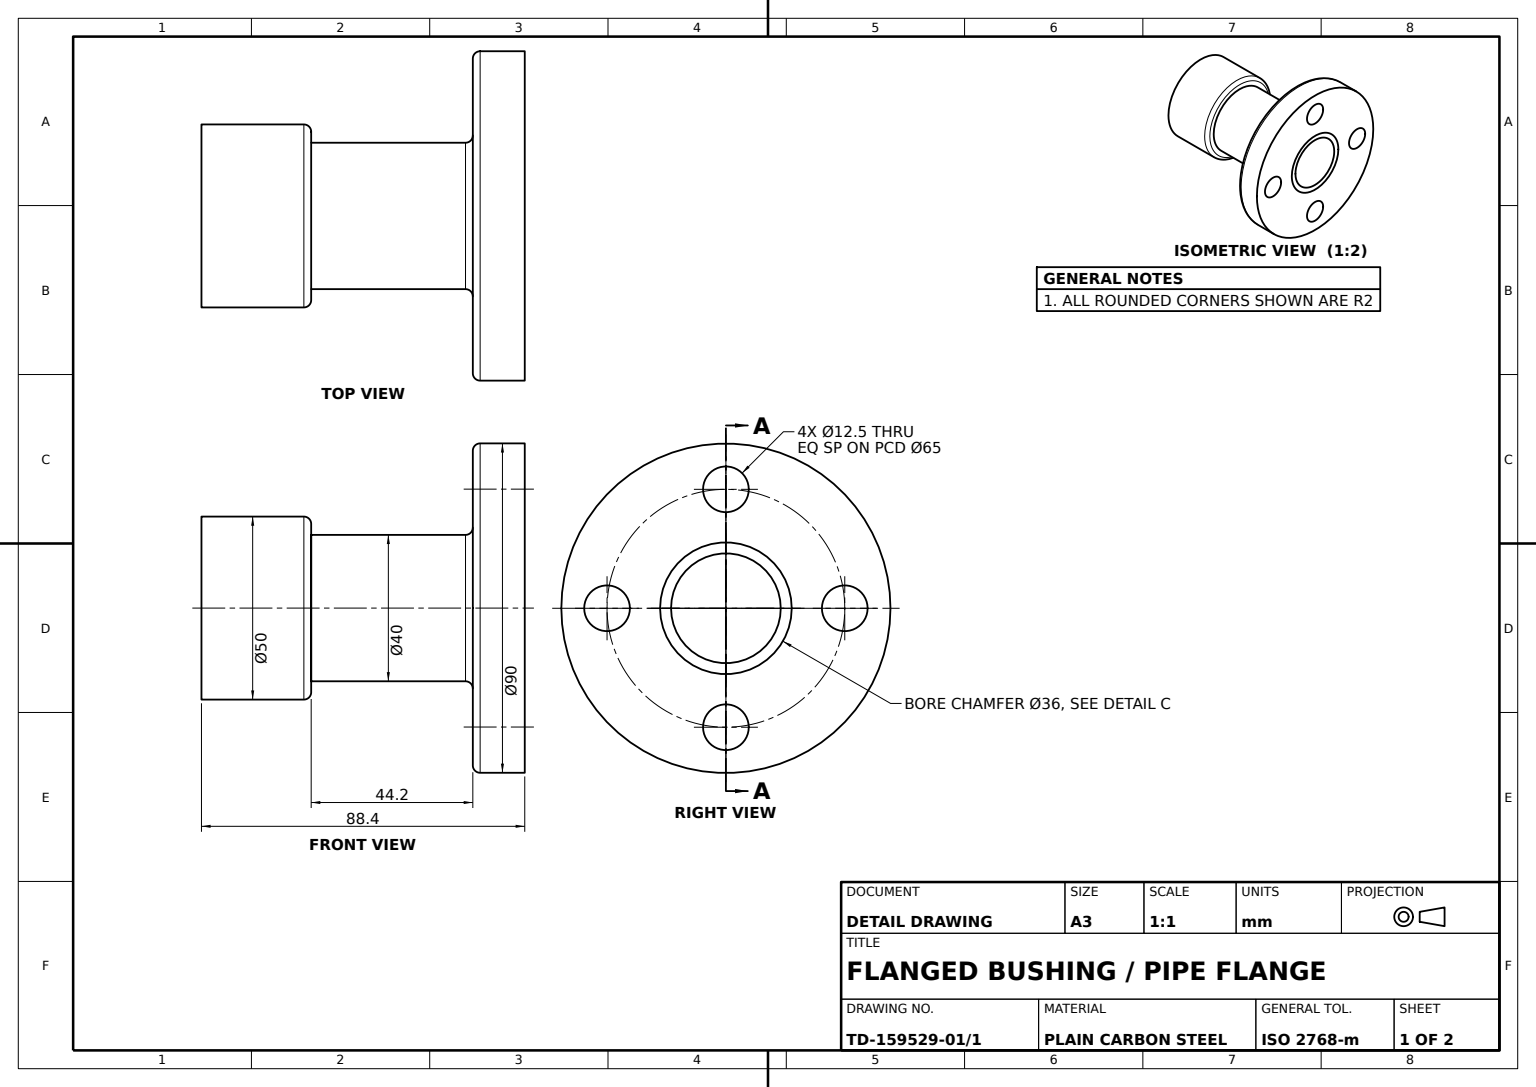
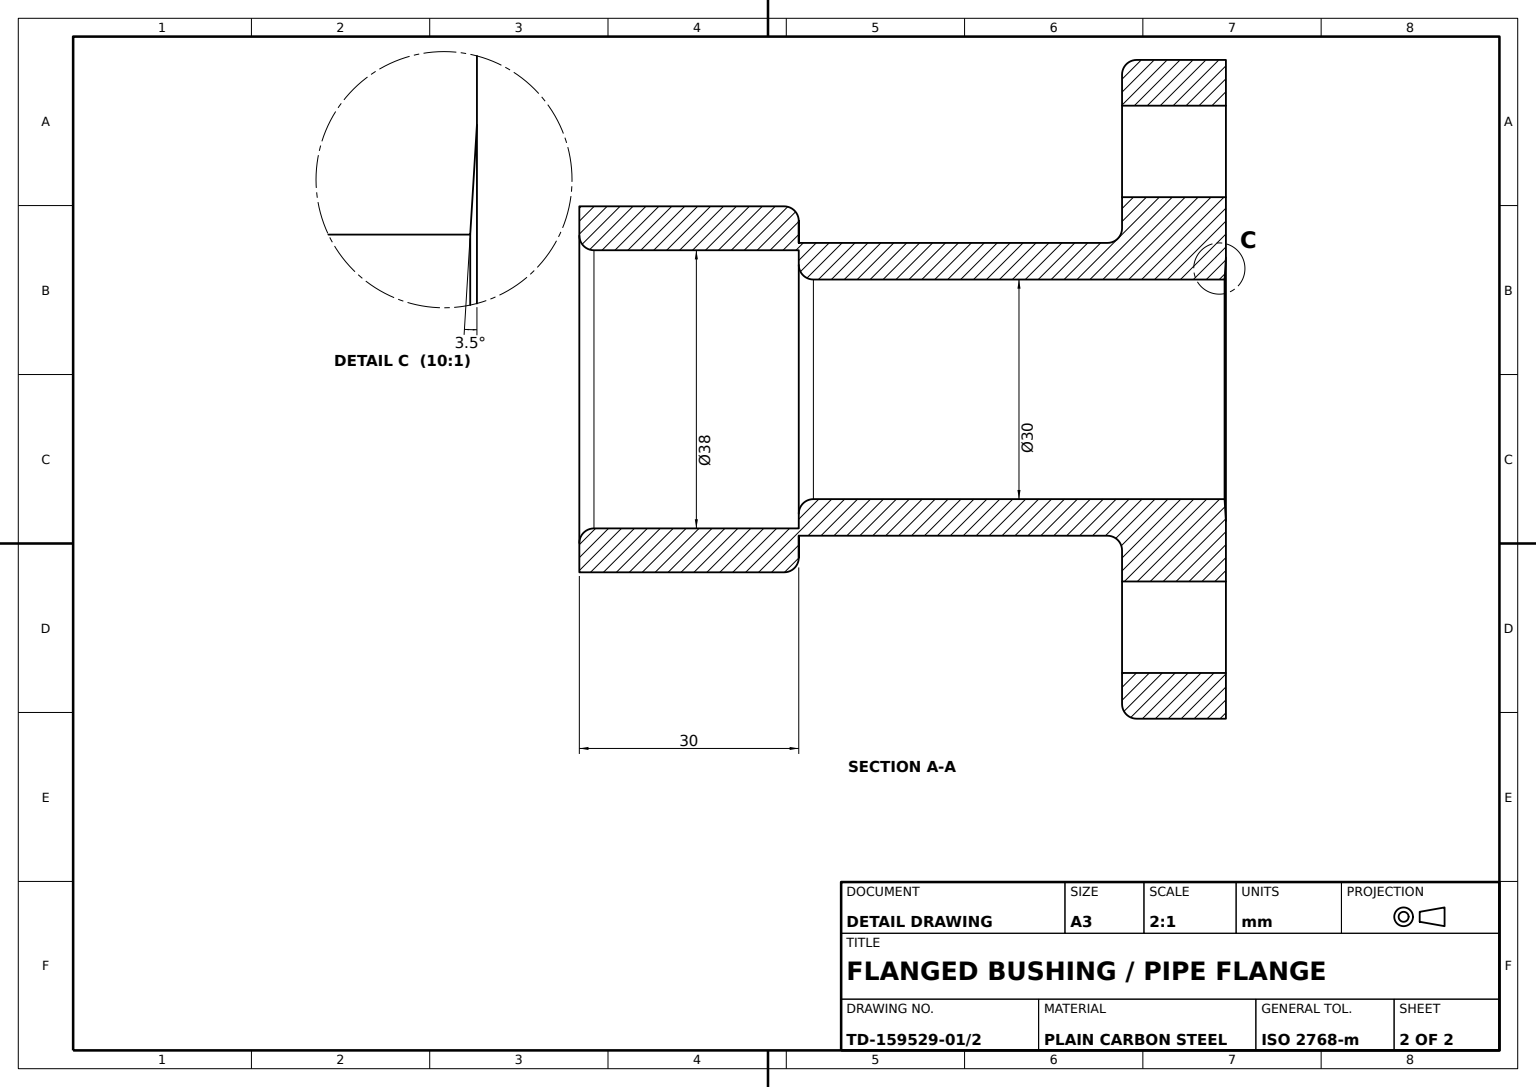
SolidWorks part; units mm, degrees
material "Plain Carbon Steel"
ref_plane "Front Plane" through (0, 0, 0) normal (0, 0, 1) x (1, 0, 0)
ref_plane "Top Plane" through (0, 0, 0) normal (0, 1, 0) x (1, 0, 0)
ref_plane "Right Plane" through (0, 0, 0) normal (1, 0, 0) x (0, 0, -1)
sketch "Flange Profile Ø90" plane through (0, 0, 0) normal (0, 0, 1) x (1, 0, 0)
  circle A0 centre (0, 0) radius 45
  dimension "D1" = 90
extrude "Flange Ø90" add sketch "Flange Profile Ø90" along normal blind 14.2
sketch "Flange Holes Sketch" plane through (0, 0, 14.2) normal (0, 0, 1) x (1, 0, 0)
  line L0 (-65.0046, 0) -> (69.5311, 0) construction
  line L1 (0, 22.0435) -> (0, -8.0721) construction
  circle A0 centre (0, 32.5) radius 6.25
  circle A1 centre (0, -32.5) radius 6.25
  circle A2 centre (-32.5, 0) radius 6.25
  circle A3 centre (32.5, 0) radius 6.25
  dimension "D1" = 12.5
  dimension "D2" = 12.5
  dimension "D5" = 12.5
  dimension "D6" = 12.5
  dimension "D3" = 65
  dimension "D4" = 32.5
  dimension "65" = 65
extrude "Flange Holes 4xØ12.5" cut sketch "Flange Holes Sketch" against normal blind 14.2
sketch "Shank Profile Ø40" plane through (0, 0, 14.2) normal (0, 0, 1) x (1, 0, 0)
  circle A0 centre (0, 0) radius 20
  dimension "D1" = 40
extrude "Shank Ø40" add sketch "Shank Profile Ø40" along normal blind 44.2
sketch "Bore Profile Ø30" plane through (0, 0, 0) normal (0, 0, -1) x (-1, 0, 0)
  circle A0 centre (0, 0) radius 15
  dimension "D1" = 30
extrude "Through Bore Ø30" cut sketch "Bore Profile Ø30" against normal through all
chamfer "Bore Chamfer 3mm" distance 3 angle 3.5 1 edges at (-15, 0, 0)
sketch "Collar Profile Ø50-Ø38" plane through (0, 0, 58.4) normal (0, 0, 1) x (1, 0, 0)
  circle A0 centre (0, 0) radius 25
  circle A1 centre (0, 0) radius 19
  dimension "D1" = 50
  dimension "D2" = 38
extrude "End Collar Ø50" add sketch "Collar Profile Ø50-Ø38" along normal blind 30
fillet "Flange Edge Fillet R2" radius 2 1 edges at (45, 0, 14.2)
fillet "Flange-Shank Fillet R2" radius 2 1 edges at (20, 0, 14.2)
fillet "Collar Fillet R2 A" radius 2 1 edges at (19, 0, 88.4)
fillet "Shank Bore Fillet R2" radius 2 1 edges at (-15, 0, 58.4)
fillet "Collar Fillet R2 B" radius 2 1 edges at (25, 0, 58.4)
